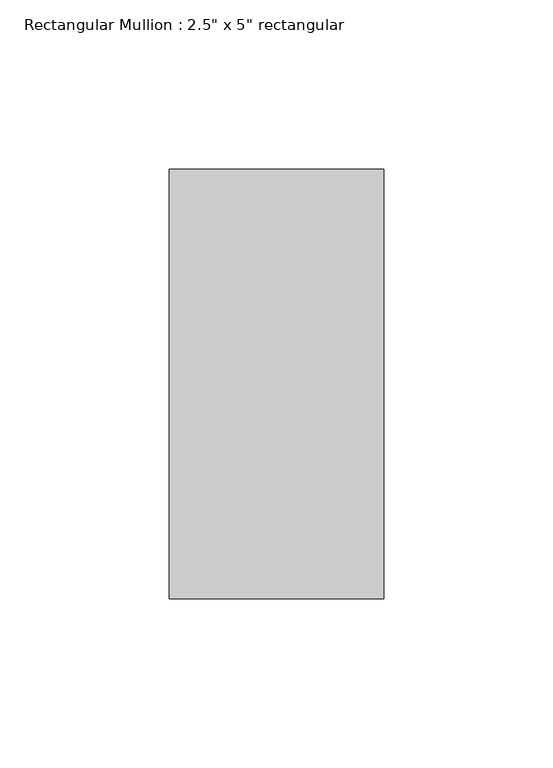
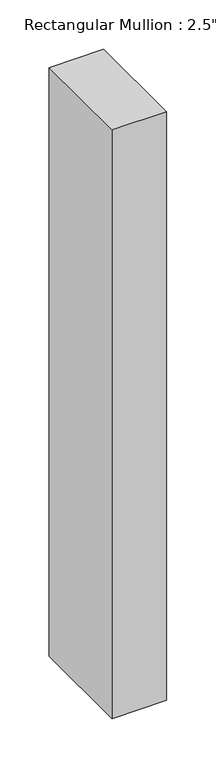
"""IFC4 building model written with IfcOpenShell, lengths in millimetres: member geometry."""

from ifc_helpers import new_model, si_unit, frame, origin, place, context, project, spatial, polyline, outline, extrude, source, transform, mapped, element, save


def member_ea9411ea(model_context):
    return source(origin(), model_context, "Body", "SweptSolid", [
        extrude(outline(polyline([(0.0, 63.5), (0.0, -63.5), (-63.5, -63.5), (-63.5, 63.5), (0.0, 63.5)])), frame((0.0, 0.0, -726.0166667), z_axis=(0.0, 0.0, 1.0), x_axis=(1.0, 0.0, 0.0)), (0.0, 0.0, 1.0), 726.0166667),
    ])


if __name__ == "__main__":
    model = new_model("IFC4")
    model_context = context("Model", 3, world=origin())
    ifc_project = project(units=[si_unit("LENGTHUNIT", "METRE", prefix="MILLI")], contexts=[model_context])
    site = spatial("IfcSite", under=ifc_project)
    building = spatial("IfcBuilding", under=site)
    placement = place(None, origin())
    member_shape = member_ea9411ea(model_context)
    element("IfcMember", 1, ObjectType="Rectangular Mullion : 2.5\" x 5\" rectangular", at=placement, inside=building, context=model_context, shape_type="MappedRepresentation", body=[
        mapped(member_shape, transform((0.0, 0.0, 0.0), x_axis=(1.0, 0.0, 0.0), y_axis=(0.0, 1.0, 0.0), z_axis=(0.0, 0.0, 1.0))),
    ])
    save(model, "model.ifc")

# Revit data of these elements
# Type "Rectangular Mullion : 2.5\" x 5\" rectangular"
#   built-in parameter 1007304 = 0.416667 (stored number, unit not read)
#   built-in parameter 1007301 = 0.104167 (stored number, unit not read)
#   built-in parameter 1007300 = 0.104167 (stored number, unit not read)
# Element 1 (IfcMember, "Rectangular Mullion : 2.5\" x 5\" rectangular")
#   Materials on its faces: "Aluminum"
# Materials
#   "Aluminum": class "Metal", colour RGB 247 247 247, transparency 0, Description = "Aluminum 6061", Cost = 0
